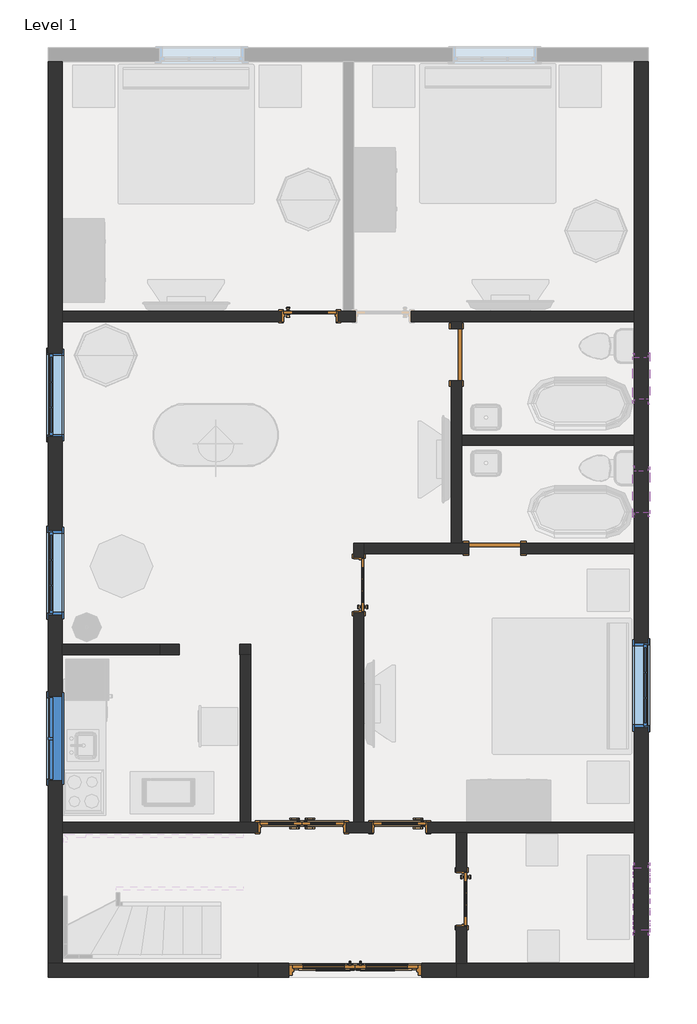
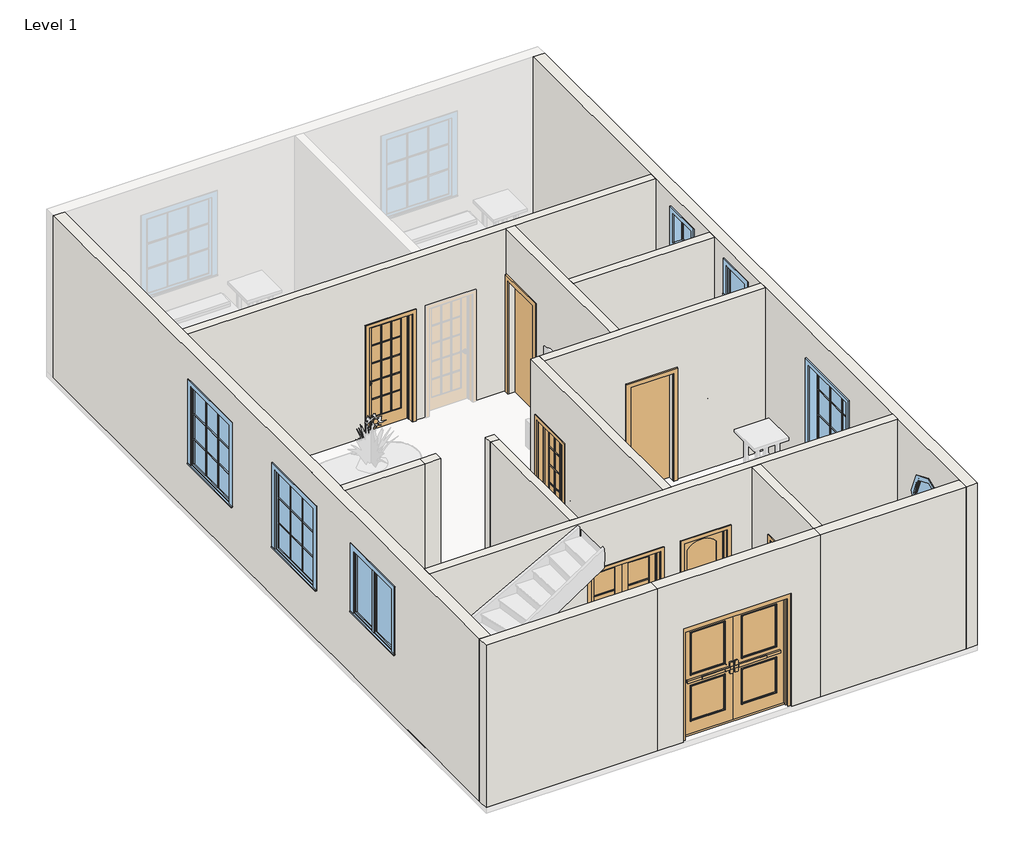
# One storey, part 1 of 2: 16 walls, 8 doors, 7 windows.
"""IFC4 building model written with IfcOpenShell, lengths in millimetres."""

from ifc_helpers import new_model, si_unit, frame, origin, origin_with_axes, place, context, project, spatial, polyline, circle_curve, outline, extrude, faceted_brep, transform, mapped, element, save
from ifc_brep_helpers import plane_surface, revolved_surface, advanced_brep
from components import door_14b9be53, door_3efe7946, door_80c43283, door_cb6735bc, door_2f28d345, door_a0b5ff2a, door_fa41f557, door_255cab33, door_e2b13fe9, window_cfa1ffdd, window_0862ab64, window_736d8d37, window_e41d21a6

model = new_model("IFC4")

# Units and contexts
model_context = context("Model", 3, world=origin())
ifc_project = project(units=[si_unit("LENGTHUNIT", "METRE", prefix="MILLI")], contexts=[model_context])

# Site, building, storey
site = spatial("IfcSite", under=ifc_project)
building = spatial("IfcBuilding", under=site)
storey = spatial("IfcBuildingStorey", under=building, Name="Level 1", Elevation=0.0)

# Doors
placement = place(None, origin())
door_shape = door_14b9be53(model_context)
element("IfcDoor", 1, ObjectType="30\" x 80\"", at=placement, inside=storey, context=model_context, shape_type="MappedRepresentation", body=[
    mapped(door_shape, transform((-4100.3653968, 878.6047533, 0.0), x_axis=(1.0, 0.0, 0.0), y_axis=(0.0, 1.0, 0.0), z_axis=(0.0, 0.0, 1.0))),
])
door_2_shape = door_3efe7946(model_context)
element("IfcDoor", 2, ObjectType="Door-Exterior-Double-Full Glass-Wood_Clad : 48\" x 80\"", at=placement, inside=storey, context=model_context, shape_type="MappedRepresentation", body=[
    mapped(door_2_shape, transform((-5522.7653968, 878.6047533, 0.0), x_axis=(1.0, 0.0, 0.0), y_axis=(0.0, 1.0, 0.0), z_axis=(0.0, 0.0, 1.0))),
])
door_3_shape = door_80c43283(model_context)
door_4_shape = door_cb6735bc(model_context)
door_5_shape = door_2f28d345(model_context)
element("IfcDoor", 3, ObjectType="Door-Exterior-Double-Two_Lite : 72\" x 80\"", at=placement, inside=storey, context=model_context, shape_type="MappedRepresentation", body=[
    mapped(door_3_shape, transform((-4748.0653968, -1213.7202467, 0.0), x_axis=(1.0, 0.0, 0.0), y_axis=(0.0, 1.0, 0.0), z_axis=(0.0, 0.0, 1.0))),
    mapped(door_4_shape, transform((-4748.0653968, -1213.7202467, 0.0), x_axis=(1.0, 0.0, 0.0), y_axis=(0.0, 1.0, 0.0), z_axis=(0.0, 0.0, 1.0))),
    mapped(door_5_shape, transform((-4748.0653968, -1213.7202467, 0.0), x_axis=(1.0, 0.0, 0.0), y_axis=(0.0, 1.0, 0.0), z_axis=(0.0, 0.0, 1.0))),
])
door_6_shape = door_a0b5ff2a(model_context)
element("IfcDoor", 4, ObjectType="Door-Interior-Single-Full Glass-Wood : 30\" x 80\"", at=placement, inside=storey, context=model_context, shape_type="MappedRepresentation", body=[
    mapped(door_6_shape, transform((-4694.0903968, 4406.0297533, 0.0), x_axis=(0.0, 1.0, 0.0), y_axis=(-1.0, 0.0, 0.0), z_axis=(0.0, 0.0, 1.0))),
])
door_7_shape = door_fa41f557(model_context)
element("IfcDoor", 5, ObjectType="Door-Interior-Single-Full Glass-Wood : 30\" x 80\"", at=placement, inside=storey, context=model_context, shape_type="MappedRepresentation", body=[
    mapped(door_7_shape, transform((-3195.4903968, -165.9702467, 0.0), x_axis=(0.0, -1.0, 0.0), y_axis=(1.0, 0.0, 0.0), z_axis=(0.0, 0.0, 1.0))),
])
element("IfcDoor", 6, ObjectType="Door-Interior-Single-Full Glass-Wood : 30\" x 80\"", at=placement, inside=storey, context=model_context, shape_type="MappedRepresentation", body=[
    mapped(door_7_shape, transform((-5408.4653968, 8320.8047533, 0.0), x_axis=(1.0, 0.0, 0.0), y_axis=(0.0, 1.0, 0.0), z_axis=(0.0, 0.0, 1.0))),
])
door_8_shape = door_255cab33(model_context)
element("IfcDoor", 7, ObjectType="Single-Flush : 30\" x 80\"", at=placement, inside=storey, context=model_context, shape_type="MappedRepresentation", body=[
    mapped(door_8_shape, transform((-2716.0653968, 4939.4297533, 0.0), x_axis=(-1.0, 0.0, 0.0), y_axis=(0.0, -1.0, 0.0), z_axis=(0.0, 0.0, 1.0))),
])
door_9_shape = door_e2b13fe9(model_context)
element("IfcDoor", 8, ObjectType="Single-Flush : 30\" x 84\"", at=placement, inside=storey, context=model_context, shape_type="MappedRepresentation", body=[
    mapped(door_9_shape, transform((-3274.8653968, 7758.8297533, 0.0), x_axis=(0.0, 1.0, 0.0), y_axis=(-1.0, 0.0, 0.0), z_axis=(0.0, 0.0, 1.0))),
])

# Walls
element("IfcWall", 9, ObjectType="Generic - 8\"", at=placement, inside=storey, context=model_context, shape_type="AdvancedBrep", body=[
    advanced_brep(
    [(-684.0653968, 12026.0297533, 0.0), (-684.0653968, 8393.8297533, 0.0), (-684.0653968, 8241.4297533, 0.0), (-684.0653968, 6590.4297533, 0.0), (-684.0653968, 6438.0297533, 0.0), (-684.0653968, 5015.6297533, 0.0), (-684.0653968, 4863.2297533, 0.0), (-684.0653968, 951.6297533, 0.0), (-684.0653968, 799.2297533, 0.0), (-684.0653968, -1105.7702467, 0.0), (-684.0653968, -1308.9702467, 0.0), (-684.0653968, -1308.9702467, 3048.0), (-684.0653968, -1105.7702467, 3048.0), (-684.0653968, 799.2297533, 3048.0), (-684.0653968, 951.6297533, 3048.0), (-684.0653968, 4863.2297533, 3048.0), (-684.0653968, 5015.6297533, 3048.0), (-684.0653968, 6438.0297533, 3048.0), (-684.0653968, 6590.4297533, 3048.0), (-684.0653968, 8241.4297533, 3048.0), (-684.0653968, 8393.8297533, 3048.0), (-684.0653968, 12026.0297533, 3048.0), (-684.0653968, 2335.9297533, 2438.4), (-684.0653968, 2335.9297533, 914.4), (-684.0653968, 3555.1297533, 914.4), (-684.0653968, 3555.1297533, 2438.4), (-684.0653968, 6069.7297533, 2768.6), (-684.0653968, 5460.1297533, 2768.6), (-684.0653968, 5460.1297533, 2159.0), (-684.0653968, 6069.7297533, 2159.0), (-684.0653968, 7111.1297533, 2768.6), (-684.0653968, 7111.1297533, 2159.0), (-684.0653968, 7720.7297533, 2159.0), (-684.0653968, 7720.7297533, 2768.6), (-684.0653968, -623.1702467, 1981.2), (-684.0653968, 291.2297533, 1981.2), (-480.8653968, 12026.0297533, 0.0), (-480.8653968, 12026.0297533, 3048.0), (-480.8653968, -1308.9702467, 3048.0), (-480.8653968, -1308.9702467, 0.0), (-480.8653968, 2335.9297533, 2438.4), (-480.8653968, 3555.1297533, 2438.4), (-480.8653968, 3555.1297533, 914.4), (-480.8653968, 2335.9297533, 914.4), (-480.8653968, 6069.7297533, 2768.6), (-480.8653968, 6069.7297533, 2159.0), (-480.8653968, 5460.1297533, 2159.0), (-480.8653968, 5460.1297533, 2768.6), (-480.8653968, 7111.1297533, 2768.6), (-480.8653968, 7720.7297533, 2768.6), (-480.8653968, 7720.7297533, 2159.0), (-480.8653968, 7111.1297533, 2159.0), (-480.8653968, -623.1702467, 1981.2), (-480.8653968, 291.2297533, 1981.2)],
    [
        (0, 1),
        (1, 2),
        (2, 3),
        (3, 4),
        (4, 5),
        (5, 6),
        (6, 7),
        (7, 8),
        (8, 9),
        (9, 10),
        (10, 11),
        (11, 12),
        (12, 13),
        (13, 14),
        (14, 15),
        (15, 16),
        (16, 17),
        (17, 18),
        (18, 19),
        (19, 20),
        (20, 21),
        (21, 0),
        (22, 23),
        (23, 24),
        (24, 25),
        (25, 22),
        (26, 27),
        (27, 28),
        (28, 29),
        (29, 26),
        (30, 31),
        (31, 32),
        (32, 33),
        (33, 30),
        (34, 35, circle_curve(frame((-684.0653968, -165.9702467, 1981.2), z_axis=(1.0, 0.0, 0.0), x_axis=(0.0, 1.0, 0.0)), 457.2)),
        (35, 34, circle_curve(frame((-684.0653968, -165.9702467, 1981.2), z_axis=(1.0, 0.0, 0.0), x_axis=(0.0, 1.0, 0.0)), 457.2)),
        (36, 37),
        (37, 38),
        (38, 39),
        (39, 36),
        (40, 41),
        (41, 42),
        (42, 43),
        (43, 40),
        (44, 45),
        (45, 46),
        (46, 47),
        (47, 44),
        (48, 49),
        (49, 50),
        (50, 51),
        (51, 48),
        (52, 53, circle_curve(frame((-480.8653968, -165.9702467, 1981.2), z_axis=(-1.0, 0.0, 0.0), x_axis=(0.0, 1.0, 0.0)), 457.2)),
        (53, 52, circle_curve(frame((-480.8653968, -165.9702467, 1981.2), z_axis=(-1.0, 0.0, 0.0), x_axis=(0.0, 1.0, 0.0)), 457.2)),
        (0, 36),
        (39, 10),
        (21, 37),
        (38, 11),
        (22, 40),
        (43, 23),
        (42, 24),
        (41, 25),
        (44, 26),
        (29, 45),
        (28, 46),
        (27, 47),
        (30, 48),
        (51, 31),
        (50, 32),
        (49, 33),
        (34, 52),
        (53, 35),
    ],
    [
        plane_surface(frame((-684.0653968, 12127.6297533, 0.0), z_axis=(-1.0, 0.0, 0.0), x_axis=(0.0, -1.0, 0.0))),
        plane_surface(frame((-480.8653968, 12127.6297533, 0.0), z_axis=(1.0, 0.0, 0.0), x_axis=(0.0, 1.0, 0.0))),
        plane_surface(frame((-684.0653968, 12127.6297533, 0.0), z_axis=(0.0, 0.0, -1.0), x_axis=(1.0, 0.0, 0.0))),
        plane_surface(frame((-9116.8653968, 12026.0297533, 0.0), z_axis=(0.0, 1.0, 0.0), x_axis=(1.0, 0.0, 0.0))),
        plane_surface(frame((-582.4653968, -1308.9702467, 0.0), z_axis=(0.0, -1.0, 0.0), x_axis=(1.0, 0.0, 0.0))),
        plane_surface(frame((-684.0653968, 2335.9297533, 2438.4), z_axis=(0.0, 1.0, 0.0), x_axis=(1.0, 0.0, 0.0))),
        plane_surface(frame((-684.0653968, 2335.9297533, 914.4), z_axis=(0.0, 0.0, 1.0), x_axis=(1.0, 0.0, 0.0))),
        plane_surface(frame((-684.0653968, 3555.1297533, 914.4), z_axis=(0.0, -1.0, 0.0), x_axis=(1.0, 0.0, 0.0))),
        plane_surface(frame((-684.0653968, 3555.1297533, 2438.4), z_axis=(0.0, 0.0, -1.0), x_axis=(1.0, 0.0, 0.0))),
        plane_surface(frame((-480.8653968, 6069.7297533, 2768.6), z_axis=(0.0, -1.0, 0.0), x_axis=(-1.0, 0.0, 0.0))),
        plane_surface(frame((-480.8653968, 6069.7297533, 2159.0), z_axis=(0.0, 0.0, 1.0), x_axis=(-1.0, 0.0, 0.0))),
        plane_surface(frame((-480.8653968, 5460.1297533, 2159.0), z_axis=(0.0, 1.0, 0.0), x_axis=(-1.0, 0.0, 0.0))),
        plane_surface(frame((-480.8653968, 5460.1297533, 2768.6), z_axis=(0.0, 0.0, -1.0), x_axis=(-1.0, 0.0, 0.0))),
        plane_surface(frame((-684.0653968, 7111.1297533, 2768.6), z_axis=(0.0, 1.0, 0.0), x_axis=(1.0, 0.0, 0.0))),
        plane_surface(frame((-684.0653968, 7111.1297533, 2159.0), z_axis=(0.0, 0.0, 1.0), x_axis=(1.0, 0.0, 0.0))),
        plane_surface(frame((-684.0653968, 7720.7297533, 2159.0), z_axis=(0.0, -1.0, 0.0), x_axis=(1.0, 0.0, 0.0))),
        plane_surface(frame((-684.0653968, 7720.7297533, 2768.6), z_axis=(0.0, 0.0, -1.0), x_axis=(1.0, 0.0, 0.0))),
        revolved_surface(polyline([(-480.8653968, 291.22975329999997, 1981.2), (-684.0653968, 291.22975329999997, 1981.2)]), (-480.8653968, -165.9702467, 1981.2), (1.0, 0.0, 0.0)),
        plane_surface(frame((-480.8653968, -1308.9702467, 3048.0), z_axis=(0.0, 0.0, 1.0), x_axis=(1.0, 0.0, 0.0))),
    ],
    [
        (0, [[1, 2, 3, 4, 5, 6, 7, 8, 9, 10, 11, 12, 13, 14, 15, 16, 17, 18, 19, 20, 21, 22], [23, 24, 25, 26], [27, 28, 29, 30], [31, 32, 33, 34], [35, 36]]),
        (1, [[37, 38, 39, 40], [41, 42, 43, 44], [45, 46, 47, 48], [49, 50, 51, 52], [53, 54]]),
        (2, [[-10, -9, -8, -7, -6, -5, -4, -3, -2, -1, 55, -40, 56]]),
        (3, [[-22, 57, -37, -55]]),
        (4, [[-11, -56, -39, 58]]),
        (5, [[-23, 59, -44, 60]]),
        (6, [[-24, -60, -43, 61]]),
        (7, [[-25, -61, -42, 62]]),
        (8, [[-26, -62, -41, -59]]),
        (9, [[-45, 63, -30, 64]]),
        (10, [[-46, -64, -29, 65]]),
        (11, [[-47, -65, -28, 66]]),
        (12, [[-48, -66, -27, -63]]),
        (13, [[-31, 67, -52, 68]]),
        (14, [[-32, -68, -51, 69]]),
        (15, [[-33, -69, -50, 70]]),
        (16, [[-34, -70, -49, -67]]),
        (17, [[-35, 71, -54, 72]]),
        (17, [[-36, -72, -53, -71]]),
        (18, [[-21, -20, -19, -18, -17, -16, -15, -14, -13, -12, -58, -38, -57]]),
    ],
),
])
element("IfcWall", 10, ObjectType="Generic - 8\"", at=placement, inside=storey, context=model_context, shape_type="Brep", body=[
    faceted_brep([(-684.0653968, -1105.7702467, 0.0), (-3122.4653968, -1105.7702467, 0.0), (-3274.8653968, -1105.7702467, 0.0), (-3274.8653968, -1105.7702467, 3048.0), (-3122.4653968, -1105.7702467, 3048.0), (-684.0653968, -1105.7702467, 3048.0), (-684.0653968, -1308.9702467, 0.0), (-684.0653968, -1308.9702467, 3048.0), (-3274.8653968, -1308.9702467, 3048.0), (-3274.8653968, -1308.9702467, 0.0)], [[[0, 1, 2, 3, 4, 5]], [[6, 7, 8, 9]], [[2, 1, 0, 6, 9]], [[0, 5, 7, 6]], [[3, 2, 9, 8]], [[5, 4, 3, 8, 7]]]),
])
element("IfcWall", 11, ObjectType="Generic - 8\"", at=placement, inside=storey, context=model_context, shape_type="Brep", body=[
    faceted_brep([(-9015.2653968, -1105.7702467, 0.0), (-9015.2653968, 799.2297533, 0.0), (-9015.2653968, 951.6297533, 0.0), (-9015.2653968, 3390.0297533, 0.0), (-9015.2653968, 3542.4297533, 0.0), (-9015.2653968, 8241.4297533, 0.0), (-9015.2653968, 8393.8297533, 0.0), (-9015.2653968, 12026.0297533, 0.0), (-9015.2653968, 12026.0297533, 3048.0), (-9015.2653968, 8393.8297533, 3048.0), (-9015.2653968, 8241.4297533, 3048.0), (-9015.2653968, 3542.4297533, 3048.0), (-9015.2653968, 3390.0297533, 3048.0), (-9015.2653968, 951.6297533, 3048.0), (-9015.2653968, 799.2297533, 3048.0), (-9015.2653968, -1105.7702467, 3048.0), (-9015.2653968, 7784.2297533, 2438.4), (-9015.2653968, 7784.2297533, 914.4), (-9015.2653968, 6565.0297533, 914.4), (-9015.2653968, 6565.0297533, 2438.4), (-9015.2653968, 5193.4297533, 2438.4), (-9015.2653968, 5193.4297533, 914.4), (-9015.2653968, 3974.2297533, 914.4), (-9015.2653968, 3974.2297533, 2438.4), (-9015.2653968, 2780.4297533, 2387.6), (-9015.2653968, 2780.4297533, 1168.4), (-9015.2653968, 1561.2297533, 1168.4), (-9015.2653968, 1561.2297533, 2387.6), (-9218.4653968, -1105.7702467, 0.0), (-9218.4653968, -1105.7702467, 3048.0), (-9218.4653968, 12026.0297533, 3048.0), (-9218.4653968, 12026.0297533, 0.0), (-9218.4653968, 7784.2297533, 2438.4), (-9218.4653968, 6565.0297533, 2438.4), (-9218.4653968, 6565.0297533, 914.4), (-9218.4653968, 7784.2297533, 914.4), (-9218.4653968, 5193.4297533, 2438.4), (-9218.4653968, 3974.2297533, 2438.4), (-9218.4653968, 3974.2297533, 914.4), (-9218.4653968, 5193.4297533, 914.4), (-9218.4653968, 2780.4297533, 2387.6), (-9218.4653968, 1561.2297533, 2387.6), (-9218.4653968, 1561.2297533, 1168.4), (-9218.4653968, 2780.4297533, 1168.4)], [[[0, 1, 2, 3, 4, 5, 6, 7, 8, 9, 10, 11, 12, 13, 14, 15], [16, 17, 18, 19], [20, 21, 22, 23], [24, 25, 26, 27]], [[28, 29, 30, 31], [32, 33, 34, 35], [36, 37, 38, 39], [40, 41, 42, 43]], [[7, 6, 5, 4, 3, 2, 1, 0, 28, 31]], [[8, 7, 31, 30]], [[0, 15, 29, 28]], [[17, 16, 32, 35]], [[18, 17, 35, 34]], [[19, 18, 34, 33]], [[16, 19, 33, 32]], [[21, 20, 36, 39]], [[22, 21, 39, 38]], [[23, 22, 38, 37]], [[20, 23, 37, 36]], [[25, 24, 40, 43]], [[26, 25, 43, 42]], [[27, 26, 42, 41]], [[24, 27, 41, 40]], [[15, 14, 13, 12, 11, 10, 9, 8, 30, 29]]]),
])
element("IfcWall", 12, ObjectType="Generic - 8\"", at=placement, inside=storey, context=model_context, shape_type="Brep", body=[
    faceted_brep([(-6170.4653968, -1105.7702467, 0.0), (-9015.2653968, -1105.7702467, 0.0), (-9218.4653968, -1105.7702467, 0.0), (-9218.4653968, -1105.7702467, 3048.0), (-9015.2653968, -1105.7702467, 3048.0), (-6170.4653968, -1105.7702467, 3048.0), (-6170.4653968, -1308.9702467, 0.0), (-6170.4653968, -1308.9702467, 3048.0), (-9218.4653968, -1308.9702467, 3048.0), (-9218.4653968, -1308.9702467, 0.0)], [[[0, 1, 2, 3, 4, 5]], [[6, 7, 8, 9]], [[2, 1, 0, 6, 9]], [[0, 5, 7, 6]], [[3, 2, 9, 8]], [[5, 4, 3, 8, 7]]]),
])
element("IfcWall", 13, ObjectType="Generic - 8\"", at=placement, inside=storey, context=model_context, shape_type="SweptSolid", body=[
    extrude(outline(polyline([(3048.0, -6170.4653968), (0.0, -6170.4653968), (0.0, -5713.2653968), (2133.6, -5713.2653968), (2133.6, -3782.8653968), (0.0, -3782.8653968), (0.0, -3274.8653968), (3048.0, -3274.8653968), (3048.0, -6170.4653968)])), frame((0.0, -1308.9702467, 0.0), z_axis=(0.0, 1.0, 0.0), x_axis=(0.0, 0.0, 1.0)), (0.0, 0.0, 1.0), 203.2),
])
element("IfcWall", 14, ObjectType="INNER WALL", at=placement, inside=storey, context=model_context, shape_type="SweptSolid", body=[
    extrude(outline(polyline([(-1105.7702467, 0.0), (-1105.7702467, 3048.0), (799.2297533, 3048.0), (799.2297533, 0.0), (240.4297533, 0.0), (240.4297533, 2057.4), (-572.3702467, 2057.4), (-572.3702467, 0.0), (-1105.7702467, 0.0)])), frame((-3274.8653968, 0.0, 0.0), z_axis=(1.0, 0.0, 0.0), x_axis=(0.0, 1.0, 0.0)), (0.0, 0.0, 1.0), 152.4),
])
element("IfcWall", 15, ObjectType="INNER WALL", at=placement, inside=storey, context=model_context, shape_type="Brep", body=[
    faceted_brep([(-684.0653968, 8241.4297533, 0.0), (-684.0653968, 8241.4297533, 3048.0), (-3198.6653968, 8241.4297533, 3048.0), (-3351.0653968, 8241.4297533, 3048.0), (-9015.2653968, 8241.4297533, 3048.0), (-9015.2653968, 8241.4297533, 0.0), (-5814.8653968, 8241.4297533, 0.0), (-5814.8653968, 8241.4297533, 2057.4), (-5002.0653968, 8241.4297533, 2057.4), (-5002.0653968, 8241.4297533, 0.0), (-4748.0653968, 8241.4297533, 0.0), (-4748.0653968, 8241.4297533, 2057.4), (-3935.2653968, 8241.4297533, 2057.4), (-3935.2653968, 8241.4297533, 0.0), (-3351.0653968, 8241.4297533, 0.0), (-3198.6653968, 8241.4297533, 0.0), (-684.0653968, 8393.8297533, 3048.0), (-684.0653968, 8393.8297533, 0.0), (-3935.2653968, 8393.8297533, 0.0), (-3935.2653968, 8393.8297533, 2057.4), (-4748.0653968, 8393.8297533, 2057.4), (-4748.0653968, 8393.8297533, 0.0), (-4773.4653968, 8393.8297533, 0.0), (-4925.8653968, 8393.8297533, 0.0), (-5002.0653968, 8393.8297533, 0.0), (-5002.0653968, 8393.8297533, 2057.4), (-5814.8653968, 8393.8297533, 2057.4), (-5814.8653968, 8393.8297533, 0.0), (-9015.2653968, 8393.8297533, 0.0), (-9015.2653968, 8393.8297533, 3048.0), (-4925.8653968, 8393.8297533, 3048.0), (-4773.4653968, 8393.8297533, 3048.0)], [[[0, 1, 2, 3, 4, 5, 6, 7, 8, 9, 10, 11, 12, 13, 14, 15]], [[16, 17, 18, 19, 20, 21, 22, 23, 24, 25, 26, 27, 28, 29, 30, 31]], [[5, 28, 27, 6]], [[17, 0, 15, 14, 13, 18]], [[9, 24, 23, 22, 21, 10]], [[1, 0, 17, 16]], [[5, 4, 29, 28]], [[8, 25, 24, 9]], [[25, 8, 7, 26]], [[26, 7, 6, 27]], [[20, 11, 10, 21]], [[11, 20, 19, 12]], [[12, 19, 18, 13]], [[4, 3, 2, 1, 16, 31, 30, 29]]]),
])
element("IfcWall", 16, ObjectType="INNER WALL", at=placement, inside=storey, context=model_context, shape_type="SweptSolid", body=[
    extrude(outline(polyline([(-7592.8653968, 3390.0297533), (-9015.2653968, 3390.0297533), (-9015.2653968, 3542.4297533), (-7592.8653968, 3542.4297533), (-7592.8653968, 3390.0297533)])), origin_with_axes(), (0.0, 0.0, 1.0), 3048.0),
])
element("IfcWall", 17, ObjectType="INNER WALL", at=placement, inside=storey, context=model_context, shape_type="SweptSolid", body=[
    extrude(outline(polyline([(-6424.4653968, 951.6297533), (-6424.4653968, 3390.0297533), (-6272.0653968, 3390.0297533), (-6272.0653968, 951.6297533), (-6424.4653968, 951.6297533)])), origin_with_axes(), (0.0, 0.0, 1.0), 3048.0),
])
element("IfcWall", 18, ObjectType="INNER WALL", at=placement, inside=storey, context=model_context, shape_type="Brep", body=[
    faceted_brep([(-6430.8153968, 3390.0297533, 0.0), (-6424.4653968, 3390.0297533, 0.0), (-6272.0653968, 3390.0297533, 0.0), (-6272.0653968, 3390.0297533, 3048.0), (-6424.4653968, 3390.0297533, 3048.0), (-6430.8153968, 3390.0297533, 3048.0), (-6430.8153968, 3542.4297533, 0.0), (-6430.8153968, 3542.4297533, 3048.0), (-6272.0653968, 3542.4297533, 3048.0), (-6272.0653968, 3542.4297533, 0.0)], [[[0, 1, 2, 3, 4, 5]], [[6, 7, 8, 9]], [[2, 1, 0, 6, 9]], [[0, 5, 7, 6]], [[3, 2, 9, 8]], [[5, 4, 3, 8, 7]]]),
])
element("IfcWall", 19, ObjectType="INNER WALL", at=placement, inside=storey, context=model_context, shape_type="Brep", body=[
    faceted_brep([(-684.0653968, 799.2297533, 0.0), (-684.0653968, 799.2297533, 3048.0), (-3122.4653968, 799.2297533, 3048.0), (-3274.8653968, 799.2297533, 3048.0), (-9015.2653968, 799.2297533, 3048.0), (-9015.2653968, 799.2297533, 0.0), (-6157.7653968, 799.2297533, 0.0), (-6157.7653968, 799.2297533, 2057.4), (-4887.7653968, 799.2297533, 2057.4), (-4887.7653968, 799.2297533, 0.0), (-4506.7653968, 799.2297533, 0.0), (-4506.7653968, 799.2297533, 2057.4), (-3693.9653968, 799.2297533, 2057.4), (-3693.9653968, 799.2297533, 0.0), (-3274.8653968, 799.2297533, 0.0), (-3122.4653968, 799.2297533, 0.0), (-684.0653968, 951.6297533, 3048.0), (-684.0653968, 951.6297533, 0.0), (-3693.9653968, 951.6297533, 0.0), (-3693.9653968, 951.6297533, 2057.4), (-4506.7653968, 951.6297533, 2057.4), (-4506.7653968, 951.6297533, 0.0), (-4621.0653968, 951.6297533, 0.0), (-4773.4653968, 951.6297533, 0.0), (-4887.7653968, 951.6297533, 0.0), (-4887.7653968, 951.6297533, 2057.4), (-6157.7653968, 951.6297533, 2057.4), (-6157.7653968, 951.6297533, 0.0), (-6272.0653968, 951.6297533, 0.0), (-6424.4653968, 951.6297533, 0.0), (-9015.2653968, 951.6297533, 0.0), (-9015.2653968, 951.6297533, 3048.0), (-6424.4653968, 951.6297533, 3048.0), (-6272.0653968, 951.6297533, 3048.0), (-4773.4653968, 951.6297533, 3048.0), (-4621.0653968, 951.6297533, 3048.0)], [[[0, 1, 2, 3, 4, 5, 6, 7, 8, 9, 10, 11, 12, 13, 14, 15]], [[16, 17, 18, 19, 20, 21, 22, 23, 24, 25, 26, 27, 28, 29, 30, 31, 32, 33, 34, 35]], [[17, 0, 15, 14, 13, 18]], [[5, 30, 29, 28, 27, 6]], [[9, 24, 23, 22, 21, 10]], [[1, 0, 17, 16]], [[5, 4, 31, 30]], [[8, 25, 24, 9]], [[25, 8, 7, 26]], [[26, 7, 6, 27]], [[12, 19, 18, 13]], [[19, 12, 11, 20]], [[20, 11, 10, 21]], [[4, 3, 2, 1, 16, 35, 34, 33, 32, 31]]]),
])
element("IfcWall", 20, ObjectType="INNER WALL", at=placement, inside=storey, context=model_context, shape_type="Brep", body=[
    faceted_brep([(-4621.0653968, 4863.2297533, 0.0), (-3097.0653968, 4863.2297533, 0.0), (-3097.0653968, 4863.2297533, 2032.0), (-2335.0653968, 4863.2297533, 2032.0), (-2335.0653968, 4863.2297533, 0.0), (-684.0653968, 4863.2297533, 0.0), (-684.0653968, 4863.2297533, 3048.0), (-4621.0653968, 4863.2297533, 3048.0), (-3097.0653968, 5015.6297533, 2032.0), (-3097.0653968, 5015.6297533, 0.0), (-3198.6653968, 5015.6297533, 0.0), (-3351.0653968, 5015.6297533, 0.0), (-4621.0653968, 5015.6297533, 0.0), (-4621.0653968, 5015.6297533, 3048.0), (-3351.0653968, 5015.6297533, 3048.0), (-3198.6653968, 5015.6297533, 3048.0), (-684.0653968, 5015.6297533, 3048.0), (-684.0653968, 5015.6297533, 0.0), (-2335.0653968, 5015.6297533, 0.0), (-2335.0653968, 5015.6297533, 2032.0)], [[[0, 1, 2, 3, 4, 5, 6, 7]], [[8, 9, 10, 11, 12, 13, 14, 15, 16, 17, 18, 19]], [[18, 17, 5, 4]], [[12, 11, 10, 9, 1, 0]], [[6, 5, 17, 16]], [[0, 7, 13, 12]], [[2, 1, 9, 8]], [[3, 2, 8, 19]], [[4, 3, 19, 18]], [[7, 6, 16, 15, 14, 13]]]),
])
element("IfcWall", 21, ObjectType="INNER WALL", at=placement, inside=storey, context=model_context, shape_type="Brep", body=[
    faceted_brep([(-4773.4653968, 5015.6297533, 3048.0), (-4773.4653968, 5015.6297533, 0.0), (-4773.4653968, 4812.4297533, 0.0), (-4773.4653968, 4812.4297533, 2057.4), (-4773.4653968, 3999.6297533, 2057.4), (-4773.4653968, 3999.6297533, 0.0), (-4773.4653968, 951.6297533, 0.0), (-4773.4653968, 951.6297533, 3048.0), (-4621.0653968, 5015.6297533, 0.0), (-4621.0653968, 5015.6297533, 3048.0), (-4621.0653968, 4863.2297533, 3048.0), (-4621.0653968, 951.6297533, 3048.0), (-4621.0653968, 951.6297533, 0.0), (-4621.0653968, 3999.6297533, 0.0), (-4621.0653968, 3999.6297533, 2057.4), (-4621.0653968, 4812.4297533, 2057.4), (-4621.0653968, 4812.4297533, 0.0), (-4621.0653968, 4863.2297533, 0.0)], [[[0, 1, 2, 3, 4, 5, 6, 7]], [[8, 9, 10, 11, 12, 13, 14, 15, 16, 17]], [[1, 8, 17, 16, 2]], [[12, 6, 5, 13]], [[1, 0, 9, 8]], [[7, 6, 12, 11]], [[15, 3, 2, 16]], [[3, 15, 14, 4]], [[4, 14, 13, 5]], [[0, 7, 11, 10, 9]]]),
])
element("IfcWall", 22, ObjectType="INNER WALL", at=placement, inside=storey, context=model_context, shape_type="SweptSolid", body=[
    extrude(outline(polyline([(-3198.6653968, 6590.4297533), (-684.0653968, 6590.4297533), (-684.0653968, 6438.0297533), (-3198.6653968, 6438.0297533), (-3198.6653968, 6590.4297533)])), origin_with_axes(), (0.0, 0.0, 1.0), 3048.0),
])
element("IfcWall", 23, ObjectType="INNER WALL", at=placement, inside=storey, context=model_context, shape_type="Brep", body=[
    faceted_brep([(-3198.6653968, 8139.8297533, 2133.6), (-3198.6653968, 8139.8297533, 0.0), (-3198.6653968, 8241.4297533, 0.0), (-3198.6653968, 8241.4297533, 3048.0), (-3198.6653968, 6590.4297533, 3048.0), (-3198.6653968, 6438.0297533, 3048.0), (-3198.6653968, 5015.6297533, 3048.0), (-3198.6653968, 5015.6297533, 0.0), (-3198.6653968, 6438.0297533, 0.0), (-3198.6653968, 6590.4297533, 0.0), (-3198.6653968, 7377.8297533, 0.0), (-3198.6653968, 7377.8297533, 2133.6), (-3351.0653968, 8241.4297533, 0.0), (-3351.0653968, 8139.8297533, 0.0), (-3351.0653968, 8139.8297533, 2133.6), (-3351.0653968, 7377.8297533, 2133.6), (-3351.0653968, 7377.8297533, 0.0), (-3351.0653968, 5015.6297533, 0.0), (-3351.0653968, 5015.6297533, 3048.0), (-3351.0653968, 8241.4297533, 3048.0)], [[[0, 1, 2, 3, 4, 5, 6, 7, 8, 9, 10, 11]], [[12, 13, 14, 15, 16, 17, 18, 19]], [[2, 1, 13, 12]], [[10, 9, 8, 7, 17, 16]], [[3, 2, 12, 19]], [[7, 6, 18, 17]], [[14, 13, 1, 0]], [[15, 14, 0, 11]], [[16, 15, 11, 10]], [[6, 5, 4, 3, 19, 18]]]),
])
element("IfcWall", 24, ObjectType="INNER WALL", at=placement, inside=storey, context=model_context, shape_type="SweptSolid", body=[
    extrude(outline(polyline([(-7313.4653968, 3390.0297533), (-7592.8653968, 3390.0297533), (-7592.8653968, 3542.4297533), (-7313.4653968, 3542.4297533), (-7313.4653968, 3390.0297533)])), origin_with_axes(), (0.0, 0.0, 1.0), 3048.0),
])

# Windows
window_shape = window_cfa1ffdd(model_context)
element("IfcWindow", 25, ObjectType="Casement 3x3 with Trim : 48\" x 60\"", at=placement, inside=storey, context=model_context, shape_type="MappedRepresentation", body=[
    mapped(window_shape, transform((-582.4653968, 2945.5297533, 304.8), x_axis=(0.0, -1.0, 0.0), y_axis=(1.0, 0.0, 0.0), z_axis=(0.0, 0.0, 1.0))),
])
element("IfcWindow", 26, ObjectType="Casement 3x3 with Trim : 48\" x 60\"", at=placement, inside=storey, context=model_context, shape_type="MappedRepresentation", body=[
    mapped(window_shape, transform((-9116.8653968, 7174.6297533, 304.8), x_axis=(0.0, 1.0, 0.0), y_axis=(-1.0, 0.0, 0.0), z_axis=(0.0, 0.0, 1.0))),
])
element("IfcWindow", 27, ObjectType="Casement 3x3 with Trim : 48\" x 60\"", at=placement, inside=storey, context=model_context, shape_type="MappedRepresentation", body=[
    mapped(window_shape, transform((-9116.8653968, 4583.8297533, 304.8), x_axis=(0.0, 1.0, 0.0), y_axis=(-1.0, 0.0, 0.0), z_axis=(0.0, 0.0, 1.0))),
])
window_2_shape = window_0862ab64(model_context)
element("IfcWindow", 28, ObjectType="Casement Dbl with Trim : 48\" x 48\"", at=placement, inside=storey, context=model_context, shape_type="MappedRepresentation", body=[
    mapped(window_2_shape, transform((-9097.8153968, 2170.8297533, 254.0), x_axis=(0.0, 1.0, 0.0), y_axis=(-1.0, 0.0, 0.0), z_axis=(0.0, 0.0, 1.0))),
])
window_3_shape = window_736d8d37(model_context)
element("IfcWindow", 29, ObjectType="Round with Trim : 36\" Diameter", at=placement, inside=storey, context=model_context, shape_type="MappedRepresentation", body=[
    mapped(window_3_shape, transform((-582.4653968, -165.9702467, 762.0), x_axis=(0.0, 1.0, 0.0), y_axis=(-1.0, 0.0, 0.0), z_axis=(0.0, 0.0, 1.0))),
])
window_4_shape = window_e41d21a6(model_context)
element("IfcWindow", 30, ObjectType="Transom with Trim : 24\" x 24\"", at=placement, inside=storey, context=model_context, shape_type="MappedRepresentation", body=[
    mapped(window_4_shape, transform((-582.4653968, 5803.0297533, 0.0), x_axis=(0.0, 1.0, 0.0), y_axis=(-1.0, 0.0, 0.0), z_axis=(0.0, 0.0, 1.0))),
])
element("IfcWindow", 31, ObjectType="Transom with Trim : 24\" x 24\"", at=placement, inside=storey, context=model_context, shape_type="MappedRepresentation", body=[
    mapped(window_4_shape, transform((-582.4653968, 7377.8297533, 0.0), x_axis=(0.0, -1.0, 0.0), y_axis=(1.0, 0.0, 0.0), z_axis=(0.0, 0.0, 1.0))),
])

save(model, "model.ifc")

# Revit data of these elements
# Type "30\" x 80\""
#   Type Mark = "9"
#   Assembly Code = "B2030100"
#   Analytic Construction = "French door, wood frame with single glass"
#   Threshold Offset [instance default] = 0' - 0 1/2"
#   Thickness = 0' - 1 3/8"
#   Thermal Resistance (R) = 1.0696 (h·ft²·°F)/BTU
#   Swing Angle [instance default] = 90.00°
#   Stiles = 0' - 4 3/4"
#   Rough Width = 2' - 8"
#   Rough Height = 6' - 9"
#   Radius = 1' - 1.00625"
#   Lock Rail = 0' - 7 1/8"
#   Height = 6' - 8"
#   Width = 2' - 6"
#   Heat Transfer Coefficient (U) = 0.9350 BTU/(h·ft²·°F)
#   Door Offset [instance default] = 0' - 0"
#   Bottom Rail = 0' - 9 1/2"
#   Threshold [instance default] = yes
#   Function = 1
#   Exterior Trim [instance default] = yes
#   Trim Material = Cherry
#   Threshold Material = Cherry
#   Panel Material = Cherry
#   Glazing = Glass
#   Frame Material = Cherry
#   Door Handle Material = Aluminum
#   Visual Light Transmittance = 0
#   Solar Heat Gain Coefficient = 0
#   Wall Closure = (empty or 0)
#   Construction Type = (empty or 0)
# Type "Door-Exterior-Double-Full Glass-Wood_Clad : 48\" x 80\""
#   Type Mark = "8"
#   Assembly Code = "B2030100"
#   Analytic Construction = "French door, wood frame with double glass"
#   Top Rail = 0' - 4 11/16"
#   Threshold Offset [instance default] = 0' - 0 1/2"
#   Thickness = 0' - 1 3/8"
#   Thermal Resistance (R) = 1.9158 (h·ft²·°F)/BTU
#   Swing Angle [instance default] = 90.00°
#   Stiles = 0' - 4 3/4"
#   Rough Width = 4' - 2"
#   Rough Height = 6' - 9"
#   Panel Width = 2' - 0"
#   Door Offset [instance default] = 0' - 0"
#   Height = 6' - 8"
#   Width = 4' - 0"
#   Heat Transfer Coefficient (U) = 0.5220 BTU/(h·ft²·°F)
#   Bottom Rail = 0' - 9 1/8"
#   Exterior Trim [instance default] = yes
#   Threshold [instance default] = yes
#   Show Grill [instance default] = yes
#   Function = 1
#   Trim Material = Cherry
#   Threshold Material = Cherry
#   Panel Material = Cherry
#   Glazing = Glass
#   Frame Material = Cherry
#   Door Handle Material = Aluminum
#   Visual Light Transmittance = 0
#   Solar Heat Gain Coefficient = 0
#   Wall Closure = (empty or 0)
#   Construction Type = (empty or 0)
# Type "Door-Exterior-Double-Two_Lite : 72\" x 80\""
#   Type Mark = "10"
#   Assembly Code = "B2030100"
#   Analytic Construction = "Metal frame, double glass door"
#   Top Rail = 0' - 4 5/8"
#   Threshold Length [instance default] = 6' - 4"
#   Threshold Offset [instance default] = 0' - 0 1/2"
#   Thickness = 0' - 1 3/4"
#   Thermal Resistance (R) = 1.3794 (h·ft²·°F)/BTU
#   Swing Angle [instance default] = 90.00°
#   Strike Height = 3' - 4"
#   Stiles = 0' - 6"
#   SinglePanelWidth = 3' - 0"
#   Rough Width [instance default] = 6' - 4"
#   Rough Height [instance default] = 7' - 0"
#   MFOpeningHeight [instance default] = 0' - 4"
#   MFOpeningWidth [instance default] = 0' - 4"
#   Lock Rail = 0' - 8"
#   Inset Calculate [instance default] = 0' - 4"
#   Masonry Inset [instance default] = 0' - 1"
#   Height = 6' - 8"
#   Width = 6' - 0"
#   Heat Transfer Coefficient (U) = 0.7250 BTU/(h·ft²·°F)
#   Glass Thickness = 0' - 0 3/4"
#   Masonry Frame Depth = 0' - 5 3/4"
#   Bottom Rail = 0' - 10"
#   Threshold [instance default] = yes
#   Masonry Frame [instance default] = yes
#   Function = 1
#   Dry Wall Frame [instance default] = no
#   Threshold Material = none
#   Panic Bar Material = Metal - Stainless Steel
#   Panel Material = Metal - Painted - Grey
#   Glass Stop Material = Metal - Painted - Grey
#   Frame Material = Metal - Painted - Grey
#   Exterior Pull Material = Metal - Stainless Steel
#   Visual Light Transmittance = 0
#   Solar Heat Gain Coefficient = 0
#   Wall Closure = (empty or 0)
# Type "Door-Interior-Single-Full Glass-Wood : 30\" x 80\""
#   Type Mark = "11"
#   Assembly Code = "C1020300"
#   Analytic Construction = "Wood frame with single clear glass"
#   Top Rail = 0' - 4 11/16"
#   Thickness = 0' - 1 3/8"
#   Thermal Resistance (R) = 1.0102 (h·ft²·°F)/BTU
#   Swing Angle [instance default] = 90.00°
#   Stiles = 0' - 4 3/4"
#   Rough Width = 2' - 8"
#   Rough Height = 6' - 9"
#   Height = 6' - 8"
#   Width = 2' - 6"
#   Heat Transfer Coefficient (U) = 0.9900 BTU/(h·ft²·°F)
#   Bottom Rail = 0' - 9 1/8"
#   Show Grill [instance default] = yes
#   Trim Material = Cherry
#   Panel Material = Cherry
#   Frame Material = Cherry
#   Door Handle Material = Aluminum
#   Visual Light Transmittance = 0
#   Solar Heat Gain Coefficient = 0
#   Wall Closure = (empty or 0)
#   Function = (empty or 0)
# Type "Single-Flush : 30\" x 80\""
#   Type Mark = "5"
#   Construction Type Id = "MDOOR"
#   Assembly Code = "C1020"
#   Analytic Construction = "Metal"
#   Thickness = 0' - 2"
#   Heat Transfer Coefficient (U) = 0.651978 BTU/(h·ft²·°F)
#   Height = 6' - 8"
#   Trim Projection Ext = 0' - 1"
#   Trim Projection Int = 0' - 1"
#   Trim Width = 0' - 3"
#   Width = 2' - 6"
#   Define Thermal Properties by = 1
#   Door Material = Door - Panel
#   Frame Material = Door - Frame
#   Visual Light Transmittance = 0
#   Solar Heat Gain Coefficient = 0
#   Function = (empty or 0)
#   Wall Closure = (empty or 0)
# Type "Single-Flush : 30\" x 84\""
#   Type Mark = "4"
#   Construction Type Id = "MDOOR"
#   Assembly Code = "C1020"
#   Analytic Construction = "Metal"
#   Thickness = 0' - 2"
#   Heat Transfer Coefficient (U) = 0.651978 BTU/(h·ft²·°F)
#   Height = 7' - 0"
#   Trim Projection Ext = 0' - 1"
#   Trim Projection Int = 0' - 1"
#   Trim Width = 0' - 3"
#   Width = 2' - 6"
#   Define Thermal Properties by = 1
#   Door Material = Door - Panel
#   Frame Material = Door - Frame
#   Visual Light Transmittance = 0
#   Solar Heat Gain Coefficient = 0
#   Function = (empty or 0)
#   Wall Closure = (empty or 0)
# Type "Generic - 8\""
#   Assembly Code = "B2010"
#   Layers, outside or top first: 0' - 8" "Brick, Common" (function 1)
# Type "INNER WALL"
#   Assembly Code = "B2010"
#   Layers, outside or top first: 0' - 6" "Brick, Common" (function 1)
# Type "Casement 3x3 with Trim : 48\" x 60\""
#   Type Mark = "11"
#   Construction Type Id = "GSP4R"
#   Assembly Code = "B2020100"
#   Analytic Construction = "1/8 in Pilkington single glazing"
#   Visual Light Transmittance = 0.9
#   Solar Heat Gain Coefficient = 0.78
#   Heat Transfer Coefficient (U) = 0.6496 BTU/(h·ft²·°F)
#   Height = 5' - 0"
#   Default Sill Height = 2' - 0"
#   Trim Projection - Ext. = 0' - 0 1/2"
#   Trim Projection - Int. = 0' - 0 3/4"
#   Trim Width - Exterior = 0' - 3 1/2"
#   Trim Width - Interior = 0' - 3 1/2"
#   Width = 4' - 0"
#   Window Inset = 0' - 0 3/4"
#   Define Thermal Properties by = 1
#   Glass Pane Material = Glass
#   Sash Material = Sash
#   Trim Exterior Material = Trim
#   Trim Interior Material = Trim
#   Wall Closure = (empty or 0)
# Type "Casement Dbl with Trim : 48\" x 48\""
#   Type Mark = "27"
#   Construction Type Id = "GSP4R"
#   Assembly Code = "B2020100"
#   Analytic Construction = "1/8 in Pilkington single glazing"
#   Visual Light Transmittance = 0.9
#   Solar Heat Gain Coefficient = 0.78
#   Heat Transfer Coefficient (U) = 0.6496 BTU/(h·ft²·°F)
#   Height = 4' - 0"
#   Default Sill Height = 3' - 0"
#   Trim Projection - Ext. = 0' - 0 1/2"
#   Trim Projection - Int. = 0' - 0 3/4"
#   Trim Width - Exterior = 0' - 3 1/2"
#   Trim Width - Interior = 0' - 3 1/2"
#   Width = 4' - 0"
#   Window Inset = 0' - 0 3/4"
#   Define Thermal Properties by = 1
#   Glass Pane Material = Glass
#   Sash Material = Sash
#   Trim Exterior Material = Trim
#   Trim Interior Material = Trim
#   Wall Closure = (empty or 0)
# Type "Round with Trim : 36\" Diameter"
#   Type Mark = "24"
#   Construction Type Id = "GSP4R"
#   Assembly Code = "B2020100"
#   Analytic Construction = "1/8 in Pilkington single glazing"
#   Visual Light Transmittance = 0.9
#   Solar Heat Gain Coefficient = 0.78
#   Heat Transfer Coefficient (U) = 0.6496 BTU/(h·ft²·°F)
#   Default Sill Height = 2' - 6"
#   Trim Projection - Ext. = 0' - 0 1/2"
#   Trim Projection - Int. = 0' - 0 3/4"
#   Trim Width - Exterior = 0' - 3 1/2"
#   Trim Width - Interior = 0' - 3 1/2"
#   Width = 3' - 0"
#   Define Thermal Properties by = 1
#   Glass Pane Material = Glass
#   Sash Material = Sash
#   Trim Exterior Material = Trim
#   Trim Interior Material = Trim
#   Wall Closure = (empty or 0)
# Type "Transom with Trim : 24\" x 24\""
#   Type Mark = "13"
#   Construction Type Id = "GSP4R"
#   Assembly Code = "B2020100"
#   Analytic Construction = "1/8 in Pilkington single glazing"
#   Visual Light Transmittance = 0.9
#   Solar Heat Gain Coefficient = 0.78
#   Heat Transfer Coefficient (U) = 0.6496 BTU/(h·ft²·°F)
#   Height = 2' - 0"
#   Default Sill Height = 7' - 1"
#   Trim Projection - Ext. = 0' - 0 1/2"
#   Trim Projection - Int. = 0' - 0 3/4"
#   Trim Width - Exterior = 0' - 3 1/2"
#   Trim Width - Interior = 0' - 3 1/2"
#   Width = 2' - 0"
#   Window Inset = 0' - 0 3/4"
#   Define Thermal Properties by = 1
#   Glass Pane Material = Glass
#   Sash Material = Sash
#   Trim Exterior Material = Trim
#   Trim Interior Material = Trim
#   Wall Closure = (empty or 0)
# Element 1 (IfcDoor, "30\" x 80\"")
#   Threshold Offset = 0' - 0 1/2"
#   Swing Angle = 90.00°
#   Door Offset = 0' - 0"
#   Threshold = yes
#   Exterior Trim = yes
#   Phase Created = New Construction
#   Materials on its faces: "Cherry", "Aluminum", "Glass"
# Element 2 (IfcDoor, "Door-Exterior-Double-Full Glass-Wood_Clad : 48\" x 80\"")
#   Threshold Offset = 0' - 0 1/2"
#   Swing Angle = 90.00°
#   Door Offset = 0' - 0"
#   Threshold = yes
#   Show Grill = yes
#   Exterior Trim = yes
#   Phase Created = New Construction
#   Materials on its faces: "Cherry", "Aluminum", "Glass"
# Element 3 (IfcDoor, "Door-Exterior-Double-Two_Lite : 72\" x 80\"")
#   Threshold Offset = 0' - 0 1/2"
#   Threshold Length = 6' - 4"
#   Swing Angle = 90.00°
#   Rough Width = 6' - 4"
#   Rough Height = 7' - 0"
#   Masonry Inset = 0' - 1"
#   MFOpeningWidth = 0' - 4"
#   MFOpeningHeight = 0' - 4"
#   Inset Calculate = 0' - 4"
#   Threshold = yes
#   Masonry Frame = yes
#   Dry Wall Frame = no
#   Phase Created = New Construction
#   Materials on its faces: "Metal - Painted - Grey", "Metal - Stainless Steel", "Glass"
# Elements 4, 5, 6 (IfcDoor, "Door-Interior-Single-Full Glass-Wood : 30\" x 80\"")
#   Swing Angle = 90.00°
#   Show Grill = yes
#   Phase Created = New Construction
#   Materials on its faces: "Cherry", "Aluminum", "Glass"
# Element 7 (IfcDoor, "Single-Flush : 30\" x 80\"")
#   Phase Created = New Construction
#   Materials on its faces: "Door - Frame", "Door - Panel"
# Element 8 (IfcDoor, "Single-Flush : 30\" x 84\"")
#   Phase Created = New Construction
#   Materials on its faces: "Door - Frame", "Door - Panel"
# Elements 9, 10, 11, 12, 13 (IfcWall, "Generic - 8\"")
#   Top Offset = 0' - 0"
#   Base Offset = 0' - 0"
#   Unconnected Height = 10' - 0"
#   wall height = 10' - 0"
#   Phase Created = New Construction
#   Base Constraint = Level 1
#   Materials on its faces: "Brick, Common"
# Elements 14, 15, 16, 17, 18, 19, 20, 21, 22, 23, 24 (IfcWall, "INNER WALL")
#   Top Offset = 0' - 0"
#   Base Offset = 0' - 0"
#   Unconnected Height = 10' - 0"
#   wall height = 10' - 0"
#   Phase Created = New Construction
#   Base Constraint = Level 1
#   Materials on its faces: "Brick, Common"
# Element 25 (IfcWindow, "Casement 3x3 with Trim : 48\" x 60\"")
#   Mark = "3"
#   Phase Created = New Construction
#   Materials on its faces: "Sash", "Glass", "Trim"
# Element 26 (IfcWindow, "Casement 3x3 with Trim : 48\" x 60\"")
#   Mark = "4"
#   Phase Created = New Construction
#   Materials on its faces: "Sash", "Glass", "Trim"
# Element 27 (IfcWindow, "Casement 3x3 with Trim : 48\" x 60\"")
#   Mark = "5"
#   Phase Created = New Construction
#   Materials on its faces: "Sash", "Glass", "Trim"
# Element 28 (IfcWindow, "Casement Dbl with Trim : 48\" x 48\"")
#   Mark = "9"
#   Phase Created = New Construction
#   Materials on its faces: "Sash", "Trim", "Glass"
# Element 29 (IfcWindow, "Round with Trim : 36\" Diameter")
#   Mark = "8"
#   Phase Created = New Construction
#   Materials on its faces: "Trim", "Sash", "Glass"
# Element 30 (IfcWindow, "Transom with Trim : 24\" x 24\"")
#   Mark = "6"
#   Phase Created = New Construction
#   Materials on its faces: "Sash", "Trim", "Glass"
# Element 31 (IfcWindow, "Transom with Trim : 24\" x 24\"")
#   Mark = "7"
#   Phase Created = New Construction
#   Materials on its faces: "Sash", "Trim", "Glass"
# Materials
#   "Cherry": class "Wood", colour RGB 226 177 128, transparency 0, Description = "Prunus Serotina", Cost = 0
#   "Glass": class "Glass", colour RGB 0 128 192, transparency 0.75, Description = "Soda Lime Glass", Cost = 0
#   "Aluminum": class "Metal", colour RGB 247 247 247, transparency 0, Description = "Aluminum 6061", Cost = 0
#   "Metal - Stainless Steel": class "Metal", colour RGB 247 247 247, transparency 0
#   "Metal - Painted - Grey": class "Paint", colour RGB 104 104 104, transparency 0, Cost = 0
#   "Door - Panel": class "Wood", colour RGB 210 159 95, transparency 0
#   "Door - Frame": colour RGB 118 70 51, transparency 0
#   "Brick, Common": class "Masonry", colour RGB 170 98 104, transparency 0, Description = "Common brick", Cost = 0
#   "Sash": class "Wood", colour RGB 224 178 126, transparency 0
#   "Trim": class "Wood", colour RGB 224 178 126, transparency 0
# Room at (-6993.143, 10453.048) mm, phase "New Construction", upper level "Level 1", upper offset 10' - 0", lower offset 0' - 0"
#   Number = "1"
#   Name = "BED ROOM"
# Room at (-2540.949, 10453.048) mm, phase "New Construction", upper level "Level 1", upper offset 10' - 0", lower offset 0' - 0"
#   Number = "2"
#   Name = "BED ROOM"
# Room at (-1792.834, 7351.109) mm, phase "New Construction", upper level "Level 1", upper offset 10' - 0", lower offset 0' - 0"
#   Number = "3"
#   Name = "Toilet"
# Room at (-1792.834, 5818.387) mm, phase "New Construction", upper level "Level 1", upper offset 10' - 0", lower offset 0' - 0"
#   Number = "4"
#   Name = "Toilet"
# Room at (-2796.403, 2862.422) mm, phase "New Construction", upper level "Level 1", upper offset 10' - 0", lower offset 0' - 0"
#   Number = "5"
#   Name = "BED ROOM"
# Room at (-1755.76, -213.829) mm, phase "New Construction", upper level "Level 1", upper offset 10' - 0", lower offset 0' - 0"
#   Number = "6"
# Room at (-7935.036, 2216.969) mm, phase "New Construction", upper level "Level 1", upper offset 10' - 0", lower offset 0' - 0"
#   Number = "7"
#   Name = "Kitchen"
# Room at (-5096.333, -213.829) mm, phase "New Construction", upper level "Level 1", upper offset 10' - 0", lower offset 0' - 0"
#   Number = "8"
#   Name = "VERANDAH"
# Room at (-6182.436, 6432.655) mm, phase "New Construction", upper level "Level 1", upper offset 10' - 0", lower offset 0' - 0"
#   Number = "9"
#   Name = "HALL AREA"
# Room at (-8221.698, 5818.387) mm, phase "New Construction", upper level "Level 1", upper offset 10' - 0", lower offset 0' - 0"
#   Number = "10"
